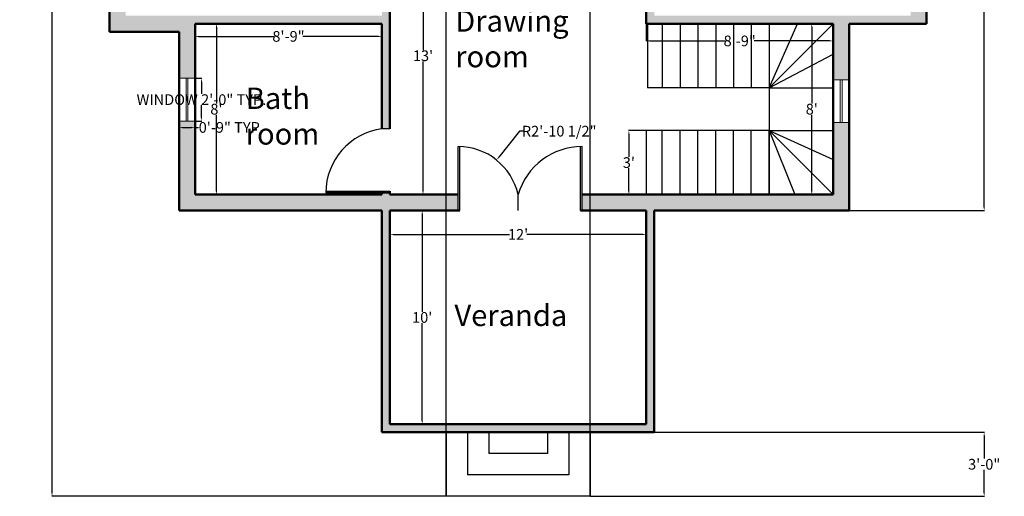
# Model space of a CAD drawing. Units: inches. Extents: x 2436 to 2989, y 5527 to 6207.
# Tile 1 of 5: x 2436 to 2989, y 5527 to 5794. Entities that reach past the tile are written whole.
import ezdxf

# ---------------------------------------------------------------- set-up
doc = ezdxf.new("R2010")
doc.units = ezdxf.units.IN
doc.header["$MEASUREMENT"] = 0
for name, color, linetype, lineweight in [('A-ANNO-DIMS', 2, 'Continuous', 18), ('A-AREA-IDEN', 7, 'Continuous', 25), ('A-DOOR', 3, 'Continuous', 25), ('A-FLOR-STRS', 7, 'Continuous', 25), ('A-GLAZ', 4, 'Continuous', 18), ('A-WALL', 7, 'Continuous', 50), ('A-WALL-PATT', 252, 'Continuous', 13)]:
    doc.layers.add(name, color=color, linetype=linetype, lineweight=lineweight)
doc.styles.get("Standard").update_dxf_attribs({"font": 'arial.ttf'})
doc.dimstyles.get("Standard").update_dxf_attribs({"dimtxt": 6, "dimasz": 2, "dimexe": 0.18, "dimexo": 0.0625, "dimgap": 0.09, "dimtad": 0, "dimtih": 1, "dimtoh": 1, "dimdec": 0, "dimzin": 0, "dimdsep": 46, "dimlunit": 3, "dimtxsty": 'Standard', "dimcen": 0.09, "dimadec": 0, "dimazin": 0, "dimtfac": 1, "dimtdec": 0, "dimtofl": 0, "dimtmove": 0, "dimatfit": 3, "dimfxl": 1, "dimtolj": 1, "dimtzin": 0, "dimarcsym": 0})

# ---------------------------------------------------------------- blocks, each defined once
blk = doc.blocks.new('*D9')
at = {"layer": 'A-ANNO-DIMS', "color": 0, "lineweight": -2, "transparency": 16777216}
for p, q in [((2534.45, 5792.23), (2546.57, 5792.23)), ((2546.39, 5790.23), (2546.39, 5747.39)), ((2546.39, 5698.23), (2546.39, 5741.08)), ((2534.45, 5696.23), (2546.57, 5696.23))]:
    blk.add_line(p, q, dxfattribs=at)
at = {"layer": 'A-ANNO-DIMS', "color": 0, "transparency": 16777216}
for points in [[(2546.05, 5790.23), (2546.72, 5790.23), (2546.39, 5792.23)], [(2546.05, 5698.23), (2546.72, 5698.23), (2546.39, 5696.23)]]:
    blk.add_solid(points, dxfattribs=at)
at = {"layer": 'Defpoints', "color": 0, "transparency": 16777216}
for p in [(2534.39, 5792.23), (2534.39, 5696.23), (2546.39, 5696.23)]:
    blk.add_point(p, dxfattribs=at)
at = {"layer": 'A-ANNO-DIMS', "color": 0, "transparency": 16777216, "insert": (2546.39, 5744.23), "char_height": 6, "attachment_point": 5}
blk.add_mtext("\\A1;8'", dxfattribs=at)
blk = doc.blocks.new('*D10')
at = {"layer": 'A-ANNO-DIMS', "color": 0, "lineweight": -2, "transparency": 16777216}
for p, q in [((2534.39, 5792.17), (2534.39, 5784.93)), ((2639.39, 5792.17), (2639.39, 5784.93)), ((2536.39, 5785.11), (2578.82, 5785.11)), ((2637.39, 5785.11), (2594.96, 5785.11))]:
    blk.add_line(p, q, dxfattribs=at)
at = {"layer": 'A-ANNO-DIMS', "color": 0, "transparency": 16777216}
for points in [[(2536.39, 5785.44), (2536.39, 5784.77), (2534.39, 5785.11)], [(2637.39, 5785.44), (2637.39, 5784.77), (2639.39, 5785.11)]]:
    blk.add_solid(points, dxfattribs=at)
at = {"layer": 'Defpoints', "color": 0, "transparency": 16777216}
for p in [(2534.39, 5792.23), (2639.39, 5792.23), (2639.39, 5785.11)]:
    blk.add_point(p, dxfattribs=at)
at = {"layer": 'A-ANNO-DIMS', "color": 0, "transparency": 16777216, "insert": (2586.89, 5785.11), "char_height": 6, "width": 15.9577, "attachment_point": 5}
blk.add_mtext('\\A1;8\'-9"', dxfattribs=at)
blk = doc.blocks.new('*D11')
at = {"layer": 'A-ANNO-DIMS', "color": 0, "lineweight": -2, "transparency": 16777216}
for p, q in [((2787.89, 5792.17), (2787.89, 5782.38)), ((2892.89, 5792.17), (2892.89, 5782.38)), ((2789.89, 5782.56), (2832.32, 5782.56)), ((2890.89, 5782.56), (2848.46, 5782.56))]:
    blk.add_line(p, q, dxfattribs=at)
at = {"layer": 'A-ANNO-DIMS', "color": 0, "transparency": 16777216}
for points in [[(2789.89, 5782.9), (2789.89, 5782.23), (2787.89, 5782.56)], [(2890.89, 5782.9), (2890.89, 5782.23), (2892.89, 5782.56)]]:
    blk.add_solid(points, dxfattribs=at)
at = {"layer": 'Defpoints', "color": 0, "transparency": 16777216}
for p in [(2787.89, 5792.23), (2892.89, 5792.23), (2892.89, 5782.56)]:
    blk.add_point(p, dxfattribs=at)
at = {"layer": 'A-ANNO-DIMS', "color": 0, "transparency": 16777216, "insert": (2840.39, 5782.56), "char_height": 6, "width": 15.9577, "attachment_point": 5}
blk.add_mtext('\\A1;8\'-9"', dxfattribs=at)
blk = doc.blocks.new('*D12')
at = {"layer": 'A-ANNO-DIMS', "color": 0, "lineweight": -2, "transparency": 16777216}
for p, q in [((2892.83, 5792.23), (2880.71, 5792.23)), ((2880.89, 5790.23), (2880.89, 5747.39)), ((2880.89, 5698.23), (2880.89, 5741.08)), ((2892.83, 5696.23), (2880.71, 5696.23))]:
    blk.add_line(p, q, dxfattribs=at)
at = {"layer": 'A-ANNO-DIMS', "color": 0, "transparency": 16777216}
for points in [[(2880.55, 5790.23), (2881.22, 5790.23), (2880.89, 5792.23)], [(2880.55, 5698.23), (2881.22, 5698.23), (2880.89, 5696.23)]]:
    blk.add_solid(points, dxfattribs=at)
at = {"layer": 'Defpoints', "color": 0, "transparency": 16777216}
for p in [(2892.89, 5792.23), (2880.89, 5696.23), (2892.89, 5696.23)]:
    blk.add_point(p, dxfattribs=at)
at = {"layer": 'A-ANNO-DIMS', "color": 0, "transparency": 16777216, "insert": (2880.89, 5744.23), "char_height": 6, "attachment_point": 5}
blk.add_mtext("\\A1;8'", dxfattribs=at)
blk = doc.blocks.new('*D13')
at = {"layer": 'A-ANNO-DIMS', "color": 0, "lineweight": -2, "transparency": 16777216}
for p, q in [((2643.95, 5852.23), (2662.66, 5852.23)), ((2662.48, 5850.23), (2662.48, 5777.39)), ((2662.48, 5698.23), (2662.48, 5771.08)), ((2643.95, 5696.23), (2662.66, 5696.23))]:
    blk.add_line(p, q, dxfattribs=at)
at = {"layer": 'A-ANNO-DIMS', "color": 0, "transparency": 16777216}
for points in [[(2662.15, 5850.23), (2662.81, 5850.23), (2662.48, 5852.23)], [(2662.15, 5698.23), (2662.81, 5698.23), (2662.48, 5696.23)]]:
    blk.add_solid(points, dxfattribs=at)
at = {"layer": 'Defpoints', "color": 0, "transparency": 16777216}
for p in [(2643.89, 5852.23), (2643.89, 5696.23), (2662.48, 5696.23)]:
    blk.add_point(p, dxfattribs=at)
at = {"layer": 'A-ANNO-DIMS', "color": 0, "transparency": 16777216, "insert": (2662.48, 5774.23), "char_height": 6, "attachment_point": 5}
blk.add_mtext("\\A1;13'", dxfattribs=at)
blk = doc.blocks.new('*D17')
at = {"layer": 'A-ANNO-DIMS', "color": 0, "lineweight": -2, "transparency": 16777216}
for p, q in [((2643.89, 5687.17), (2643.89, 5673.69)), ((2787.89, 5687.17), (2787.89, 5673.69)), ((2645.89, 5673.87), (2710.99, 5673.87)), ((2785.89, 5673.87), (2720.79, 5673.87))]:
    blk.add_line(p, q, dxfattribs=at)
at = {"layer": 'A-ANNO-DIMS', "color": 0, "transparency": 16777216}
for points in [[(2645.89, 5674.2), (2645.89, 5673.53), (2643.89, 5673.87)], [(2785.89, 5674.2), (2785.89, 5673.53), (2787.89, 5673.87)]]:
    blk.add_solid(points, dxfattribs=at)
at = {"layer": 'Defpoints', "color": 0, "transparency": 16777216}
for p in [(2643.89, 5687.23), (2787.89, 5687.23), (2787.89, 5673.87)]:
    blk.add_point(p, dxfattribs=at)
at = {"layer": 'A-ANNO-DIMS', "color": 0, "transparency": 16777216, "insert": (2715.89, 5673.87), "char_height": 6, "attachment_point": 5}
blk.add_mtext("\\A1;12'", dxfattribs=at)
blk = doc.blocks.new('*D18')
at = {"layer": 'A-ANNO-DIMS', "color": 0, "lineweight": -2, "transparency": 16777216}
for p, q in [((2643.95, 5687.23), (2662.19, 5687.23)), ((2662.01, 5685.23), (2662.01, 5630.39)), ((2662.01, 5569.23), (2662.01, 5624.08)), ((2643.95, 5567.23), (2662.19, 5567.23))]:
    blk.add_line(p, q, dxfattribs=at)
at = {"layer": 'A-ANNO-DIMS', "color": 0, "transparency": 16777216}
for points in [[(2661.68, 5685.23), (2662.34, 5685.23), (2662.01, 5687.23)], [(2661.68, 5569.23), (2662.34, 5569.23), (2662.01, 5567.23)]]:
    blk.add_solid(points, dxfattribs=at)
at = {"layer": 'Defpoints', "color": 0, "transparency": 16777216}
for p in [(2643.89, 5687.23), (2643.89, 5567.23), (2662.01, 5567.23)]:
    blk.add_point(p, dxfattribs=at)
at = {"layer": 'A-ANNO-DIMS', "color": 0, "transparency": 16777216, "insert": (2662.01, 5627.23), "char_height": 6, "attachment_point": 5}
blk.add_mtext("\\A1;10'", dxfattribs=at)
blk = doc.blocks.new('*D26')
at = {"layer": 'A-ANNO-DIMS', "color": 0, "lineweight": -2, "transparency": 16777216}
for p, q in [((2787.95, 5732.23), (2777.95, 5732.23)), ((2778.13, 5730.23), (2778.13, 5717.39)), ((2778.13, 5698.23), (2778.13, 5711.08)), ((2787.95, 5696.23), (2777.95, 5696.23))]:
    blk.add_line(p, q, dxfattribs=at)
at = {"layer": 'A-ANNO-DIMS', "color": 0, "transparency": 16777216}
for points in [[(2777.8, 5730.23), (2778.47, 5730.23), (2778.13, 5732.23)], [(2777.8, 5698.23), (2778.47, 5698.23), (2778.13, 5696.23)]]:
    blk.add_solid(points, dxfattribs=at)
at = {"layer": 'Defpoints', "color": 0, "transparency": 16777216}
for p in [(2788.02, 5732.23), (2778.13, 5696.23), (2788.02, 5696.23)]:
    blk.add_point(p, dxfattribs=at)
at = {"layer": 'A-ANNO-DIMS', "color": 0, "transparency": 16777216, "insert": (2778.13, 5714.23), "char_height": 6, "attachment_point": 5}
blk.add_mtext("\\A1;3'", dxfattribs=at)
blk = doc.blocks.new('WINDOW-24IN')
for p, q in [((0, 24), (9, 24)), ((0, 0), (0, 24)), ((4, 0), (4, 24)), ((5, 24), (5, 0)), ((9, 24), (9, 0)), ((9, 0), (0, 0))]:
    blk.add_line(p, q)
blk = doc.blocks.new('DOOR-SWING-36IN')
for p, q in [((1, 0), (1, 36)), ((1, 36), (1, 0)), ((2, 36), (2, 0)), ((0, 0), (1, 0)), ((1, 0), (2, 0)), ((37, 0), (37, 4.5))]:
    blk.add_line(p, q)
blk.add_arc((1, -0.32), 36.32, 7.6281, 90)
blk = doc.blocks.new('*D42')
at = {"layer": 'A-ANNO-DIMS', "color": 0, "lineweight": -2, "transparency": 16777216}
for p, q in [((2534.45, 5761.57), (2538.17, 5761.57)), ((2537.99, 5759.57), (2537.99, 5752.76)), ((2537.99, 5739.57), (2537.99, 5746.38)), ((2534.45, 5737.57), (2538.17, 5737.57))]:
    blk.add_line(p, q, dxfattribs=at)
at = {"layer": 'A-ANNO-DIMS', "color": 0, "transparency": 16777216}
for points in [[(2537.65, 5759.57), (2538.32, 5759.57), (2537.99, 5761.57)], [(2537.65, 5739.57), (2538.32, 5739.57), (2537.99, 5737.57)]]:
    blk.add_solid(points, dxfattribs=at)
at = {"layer": 'Defpoints', "color": 0, "transparency": 16777216}
for p in [(2534.39, 5761.57), (2537.99, 5761.57), (2534.39, 5737.57)]:
    blk.add_point(p, dxfattribs=at)
at = {"layer": 'A-ANNO-DIMS', "color": 0, "transparency": 16777216, "insert": (2537.99, 5749.57), "char_height": 6, "attachment_point": 5}
blk.add_mtext('\\A1;WINDOW 2\'-0" TYP.', dxfattribs=at)
blk = doc.blocks.new('*D43')
at = {"layer": 'A-ANNO-DIMS', "color": 0, "lineweight": -2, "transparency": 16777216}
for p, q in [((2525.39, 5737.51), (2525.39, 5733.79)), ((2534.39, 5737.51), (2534.39, 5733.79)), ((2527.39, 5733.97), (2532.39, 5733.97)), ((2534.39, 5733.97), (2536.39, 5733.97))]:
    blk.add_line(p, q, dxfattribs=at)
at = {"layer": 'A-ANNO-DIMS', "color": 0, "transparency": 16777216}
for points in [[(2527.39, 5734.3), (2527.39, 5733.64), (2525.39, 5733.97)], [(2532.39, 5734.3), (2532.39, 5733.64), (2534.39, 5733.97)]]:
    blk.add_solid(points, dxfattribs=at)
at = {"layer": 'Defpoints', "color": 0, "transparency": 16777216}
for p in [(2525.39, 5737.57), (2534.39, 5737.57), (2534.39, 5733.97)]:
    blk.add_point(p, dxfattribs=at)
at = {"layer": 'A-ANNO-DIMS', "color": 0, "transparency": 16777216, "insert": (2554.76, 5733.97), "char_height": 6, "attachment_point": 5}
blk.add_mtext('\\A1;0\'-9" TYP.', dxfattribs=at)
blk = doc.blocks.new('*D49')
at = {"layer": 'A-ANNO-DIMS', "color": 0, "lineweight": -2, "transparency": 16777216}
for p, q in [((2486.33, 6170.23), (2453.86, 6170.23)), ((2454.04, 6168.23), (2454.04, 5851.68)), ((2454.04, 5528.73), (2454.04, 5845.29)), ((2675.33, 5526.73), (2453.86, 5526.73))]:
    blk.add_line(p, q, dxfattribs=at)
at = {"layer": 'A-ANNO-DIMS', "color": 0, "transparency": 16777216}
for points in [[(2453.7, 6168.23), (2454.37, 6168.23), (2454.04, 6170.23)], [(2453.7, 5528.73), (2454.37, 5528.73), (2454.04, 5526.73)]]:
    blk.add_solid(points, dxfattribs=at)
at = {"layer": 'Defpoints', "color": 0, "transparency": 16777216}
for p in [(2486.39, 6170.23), (2454.04, 5526.73), (2675.39, 5526.73)]:
    blk.add_point(p, dxfattribs=at)
at = {"layer": 'A-ANNO-DIMS', "color": 0, "transparency": 16777216, "insert": (2454.04, 5848.48), "char_height": 6, "attachment_point": 5}
blk.add_mtext('\\A1;53\'-7 1/2"', dxfattribs=at)
blk = doc.blocks.new('*D50')
at = {"layer": 'A-ANNO-DIMS', "color": 0, "lineweight": -2, "transparency": 16777216}
for p, q in [((2792.45, 6170.23), (2977.92, 6170.23)), ((2977.74, 6168.23), (2977.74, 5931.89)), ((2977.74, 5689.23), (2977.74, 5925.58)), ((2901.95, 5687.23), (2977.92, 5687.23))]:
    blk.add_line(p, q, dxfattribs=at)
at = {"layer": 'A-ANNO-DIMS', "color": 0, "transparency": 16777216}
for points in [[(2977.4, 6168.23), (2978.07, 6168.23), (2977.74, 6170.23)], [(2977.4, 5689.23), (2978.07, 5689.23), (2977.74, 5687.23)]]:
    blk.add_solid(points, dxfattribs=at)
at = {"layer": 'Defpoints', "color": 0, "transparency": 16777216}
for p in [(2792.39, 6170.23), (2901.89, 5687.23), (2977.74, 5687.23)]:
    blk.add_point(p, dxfattribs=at)
at = {"layer": 'A-ANNO-DIMS', "color": 0, "transparency": 16777216, "insert": (2977.74, 5928.73), "char_height": 6, "attachment_point": 5}
blk.add_mtext('\\A1;40\'-3"', dxfattribs=at)
blk = doc.blocks.new('*D51')
at = {"layer": 'A-ANNO-DIMS', "color": 0, "lineweight": -2, "transparency": 16777216}
for p, q in [((2675.39, 5526.79), (2675.39, 6202.76)), ((2677.39, 6202.58), (2707.81, 6202.58)), ((2754.39, 6202.58), (2723.97, 6202.58)), ((2756.39, 5526.79), (2756.39, 6202.76))]:
    blk.add_line(p, q, dxfattribs=at)
at = {"layer": 'A-ANNO-DIMS', "color": 0, "transparency": 16777216}
for points in [[(2677.39, 6202.92), (2677.39, 6202.25), (2675.39, 6202.58)], [(2754.39, 6202.92), (2754.39, 6202.25), (2756.39, 6202.58)]]:
    blk.add_solid(points, dxfattribs=at)
at = {"layer": 'Defpoints', "color": 0, "transparency": 16777216}
for p in [(2756.39, 6202.58), (2675.39, 5526.73), (2756.39, 5526.73)]:
    blk.add_point(p, dxfattribs=at)
at = {"layer": 'A-ANNO-DIMS', "color": 0, "transparency": 16777216, "insert": (2715.89, 6202.58), "char_height": 6, "attachment_point": 5}
blk.add_mtext('\\A1;6\'-9"', dxfattribs=at)
blk = doc.blocks.new('*D52')
at = {"layer": 'A-ANNO-DIMS', "color": 0, "lineweight": -2, "transparency": 16777216}
for p, q in [((2756.45, 5562.73), (2977.92, 5562.73)), ((2977.74, 5560.73), (2977.74, 5547.89)), ((2977.74, 5528.73), (2977.74, 5541.58)), ((2756.45, 5526.73), (2977.92, 5526.73))]:
    blk.add_line(p, q, dxfattribs=at)
at = {"layer": 'A-ANNO-DIMS', "color": 0, "transparency": 16777216}
for points in [[(2977.4, 5560.73), (2978.07, 5560.73), (2977.74, 5562.73)], [(2977.4, 5528.73), (2978.07, 5528.73), (2977.74, 5526.73)]]:
    blk.add_solid(points, dxfattribs=at)
at = {"layer": 'Defpoints', "color": 0, "transparency": 16777216}
for p in [(2756.39, 5562.73), (2756.39, 5526.73), (2977.74, 5526.73)]:
    blk.add_point(p, dxfattribs=at)
at = {"layer": 'A-ANNO-DIMS', "color": 0, "transparency": 16777216, "insert": (2977.74, 5544.73), "char_height": 6, "attachment_point": 5}
blk.add_mtext('\\A1;3\'-0"', dxfattribs=at)
blk = doc.blocks.new('*D53')
at = {"layer": 'A-ANNO-DIMS', "color": 0, "lineweight": -2, "transparency": 16777216}
for p, q in [((2716.72, 5731.86), (2705, 5717.21)), ((2718.72, 5731.86), (2716.72, 5731.86)), ((2682.05, 5688.64), (2682.23, 5688.64)), ((2682.14, 5688.55), (2682.14, 5688.73))]:
    blk.add_line(p, q, dxfattribs=at)
at = {"layer": 'A-ANNO-DIMS', "color": 0, "transparency": 16777216}
blk.add_solid([(2704.74, 5717.42), (2705.26, 5717.01), (2703.75, 5715.65)], dxfattribs=at)
at = {"layer": 'Defpoints', "color": 0, "transparency": 16777216}
for p in [(2703.75, 5715.65), (2682.14, 5688.64)]:
    blk.add_point(p, dxfattribs=at)
at = {"layer": 'A-ANNO-DIMS', "color": 0, "transparency": 16777216, "insert": (2738.97, 5731.86), "char_height": 6, "attachment_point": 5}
blk.add_mtext('\\A1;R2\'-10 1/2"', dxfattribs=at)

msp = doc.modelspace()

# ---------------------------------------------------------------- hatches: boundary and pattern name
at = {"layer": 'A-WALL-PATT'}
h = msp.add_hatch(color=256, dxfattribs=at)
h.dxf.hatch_style = 1
h.paths.add_polyline_path([(2533.49, 6170.23), (2486.39, 6170.23), (2486.39, 6124.33), (2495.39, 6124.33), (2495.39, 6161.23), (2533.49, 6161.23)])
h.paths.add_polyline_path([(2677.58, 6170.23), (2593.49, 6170.23), (2593.49, 6161.23), (2639.39, 6161.23), (2639.39, 6035.73), (2639.39, 6035.73), (2643.89, 6035.73), (2643.89, 6036.73), (2685.89, 6036.73), (2685.89, 6041.23), (2643.89, 6041.23), (2643.89, 6161.23), (2677.58, 6161.23)])
h.paths.add_polyline_path([(2792.39, 6170.23), (2737.58, 6170.23), (2737.58, 6161.23), (2787.89, 6161.23), (2787.89, 6084.23), (2792.39, 6084.23), (2792.39, 6161.23), (2936.39, 6161.23), (2936.39, 6071.23), (2840.39, 6071.23), (2840.39, 6047.23), (2792.39, 6047.23), (2792.39, 6048.23), (2787.89, 6048.23), (2787.89, 6047.23), (2787.89, 6041.23), (2742.3, 6041.23), (2742.3, 6036.73), (2787.89, 6036.73), (2787.89, 6035.73), (2792.39, 6035.73), (2792.39, 6042.73), (2840.39, 6042.73), (2840.39, 5945.23), (2792.39, 5945.23), (2792.39, 6003.73), (2787.89, 6003.73), (2787.89, 5893.73), (2792.39, 5893.73), (2792.39, 5940.73), (2845.89, 5940.73), (2845.89, 5945.23), (2844.89, 5945.23), (2844.89, 6047.23), (2844.89, 6066.73), (2936.39, 6066.73), (2936.39, 6024.33), (2945.39, 6024.33), (2945.39, 6080.66), (2940.89, 6080.66), (2940.89, 6165.73), (2792.39, 6165.73)])
h.paths.add_polyline_path([(2945.39, 6000.33), (2936.39, 6000.33), (2936.39, 5945.23), (2881.89, 5945.23), (2881.89, 5940.73), (2936.39, 5940.73), (2936.39, 5901.74), (2945.39, 5901.74)], flags=17)
h.paths.add_polyline_path([(2945.39, 5841.74), (2936.39, 5841.74), (2936.39, 5796.73), (2792.39, 5796.73), (2792.39, 5857.73), (2787.89, 5857.73), (2787.89, 5856.73), (2786.89, 5856.73), (2786.89, 5852.23), (2787.89, 5852.23), (2787.89, 5792.23), (2892.89, 5792.23), (2892.89, 5760.78), (2901.89, 5760.78), (2901.89, 5792.23), (2945.39, 5792.23)])
h.paths.add_polyline_path([(2495.39, 5880.74), (2486.39, 5880.74), (2486.39, 5787.73), (2525.39, 5787.73), (2525.39, 5761.57), (2534.39, 5761.57), (2534.39, 5792.23), (2639.39, 5792.23), (2639.39, 5733.23), (2643.89, 5733.23), (2643.89, 5852.23), (2750.89, 5852.23), (2750.89, 5856.73), (2643.89, 5856.73), (2643.89, 5857.73), (2639.39, 5857.73), (2639.39, 5796.73), (2495.39, 5796.73)])
h.paths.add_polyline_path([(2495.39, 6064.33), (2486.39, 6064.33), (2486.39, 5940.74), (2495.39, 5940.74), (2495.39, 5988.73), (2639.39, 5988.73), (2639.39, 5893.73), (2643.89, 5893.73), (2643.89, 5999.73), (2639.39, 5999.73), (2639.39, 5993.23), (2495.39, 5993.23)])
h.paths.add_polyline_path([(2682.14, 5696.23), (2643.89, 5696.23), (2643.89, 5697.23), (2639.39, 5697.23), (2639.39, 5696.23), (2558.39, 5696.23), (2534.39, 5696.23), (2534.39, 5737.57), (2525.39, 5737.57), (2525.39, 5687.23), (2534.39, 5687.23), (2558.39, 5687.23), (2643.89, 5687.23), (2682.14, 5687.23)])
h.paths.add_polyline_path([(2901.89, 5736.78), (2892.89, 5736.78), (2892.89, 5696.23), (2868.89, 5696.23), (2751.89, 5696.23), (2751.89, 5687.23), (2787.89, 5687.23), (2787.89, 5567.23), (2792.39, 5567.23), (2792.39, 5687.23), (2868.89, 5687.23), (2892.89, 5687.23), (2901.89, 5687.23)])
h.paths.add_polyline_path([(2643.89, 5687.23), (2639.39, 5687.23), (2639.39, 5567.23), (2643.89, 5567.23)])
h.paths.add_polyline_path([(2787.89, 5567.23), (2643.89, 5567.23), (2643.89, 5562.73), (2787.89, 5562.73)])
h.paths.add_polyline_path([(2643.89, 5567.23), (2639.39, 5567.23), (2639.39, 5562.73), (2643.89, 5562.73)])
h.paths.add_polyline_path([(2792.39, 5567.23), (2787.89, 5567.23), (2787.89, 5562.73), (2792.39, 5562.73)])

# ---------------------------------------------------------------- linework, layer by layer
at = {"layer": 'A-DOOR'}
for p, q in [((2682.14, 5687.23), (2682.14, 5723.23)), ((2683.14, 5687.23), (2683.14, 5723.23)), ((2750.89, 5687.23), (2750.89, 5723.23)), ((2751.89, 5687.23), (2751.89, 5723.23)), ((2643.89, 5697.23), (2643.89, 5697.23)), ((2715.89, 5687.23), (2715.89, 5696.23)), ((2683.14, 5687.23), (2682.14, 5687.23)), ((2750.89, 5687.23), (2751.89, 5687.23))]:
    msp.add_line(p, q, dxfattribs=at)
for centre, radius, start, end in [((2682.14, 5688.64), 34.59, 12.6804, 90), ((2751.89, 5685.73), 37.5, 90, 163.7398)]:
    msp.add_arc(centre, radius, start, end, dxfattribs=at)
at = {"layer": 'A-FLOR-STRS'}
for p, q in [((2788.54, 5792.23), (2788.54, 5756.23)), ((2796.89, 5792.23), (2796.89, 5756.23)), ((2806.89, 5792.23), (2806.89, 5756.23)), ((2816.89, 5792.23), (2816.89, 5756.23)), ((2859.89, 5792.23), (2823.89, 5792.23)), ((2826.89, 5792.23), (2826.89, 5756.23)), ((2836.89, 5792.23), (2836.89, 5756.23)), ((2846.89, 5792.23), (2846.89, 5756.23)), ((2892.89, 5792.23), (2856.89, 5792.23)), ((2856.89, 5792.23), (2856.89, 5696.23)), ((2856.89, 5792.23), (2856.89, 5756.23)), ((2856.89, 5756.23), (2892.89, 5792.23)), ((2856.89, 5756.23), (2872.92, 5792.23)), ((2856.89, 5756.23), (2892.89, 5775.18)), ((2856.89, 5756.23), (2788.54, 5756.23)), ((2856.89, 5756.23), (2892.89, 5756.23)), ((2856.89, 5732.23), (2788.02, 5732.23)), ((2788.02, 5696.23), (2788.02, 5732.23)), ((2796.89, 5696.23), (2796.89, 5732.23)), ((2806.89, 5696.23), (2806.89, 5732.23)), ((2816.89, 5696.23), (2816.89, 5732.23)), ((2826.89, 5696.23), (2826.89, 5732.23)), ((2836.89, 5696.23), (2836.89, 5732.23)), ((2846.89, 5696.23), (2846.89, 5732.23)), ((2856.89, 5696.23), (2856.89, 5732.23)), ((2856.89, 5732.23), (2892.89, 5732.23)), ((2856.89, 5732.23), (2892.89, 5696.23)), ((2856.89, 5732.23), (2892.89, 5715.88)), ((2856.89, 5732.23), (2871.34, 5696.23)), ((2639.39, 5562.73), (2675.39, 5562.73)), ((2675.39, 5562.73), (2675.39, 5526.73)), ((2687.39, 5562.73), (2687.39, 5538.73)), ((2699.39, 5562.73), (2699.39, 5550.73)), ((2732.39, 5562.73), (2732.39, 5550.73)), ((2744.39, 5562.73), (2744.39, 5538.73)), ((2792.39, 5562.73), (2756.39, 5562.73)), ((2756.39, 5562.73), (2756.39, 5526.73)), ((2732.39, 5550.73), (2699.39, 5550.73)), ((2744.39, 5538.73), (2687.39, 5538.73)), ((2756.39, 5526.73), (2675.39, 5526.73))]:
    msp.add_line(p, q, dxfattribs=at)
at = {"layer": 'A-WALL'}
for p, q in [((2486.39, 6170.23), (2486.39, 5787.73)), ((2945.39, 6080.66), (2945.39, 5792.23)), ((2643.89, 5852.23), (2643.89, 5733.23)), ((2787.89, 5852.23), (2787.89, 5792.23)), ((2534.39, 5792.23), (2639.39, 5792.23)), ((2534.39, 5696.23), (2534.39, 5792.23)), ((2639.39, 5792.23), (2639.39, 5733.23)), ((2787.89, 5792.23), (2892.89, 5792.23)), ((2892.89, 5696.23), (2892.89, 5792.23)), ((2901.89, 5687.23), (2901.89, 5792.23)), ((2901.89, 5792.23), (2945.39, 5792.23)), ((2486.39, 5787.73), (2525.39, 5787.73)), ((2525.39, 5687.23), (2525.39, 5787.73)), ((2643.89, 5698.23), (2643.89, 5696.23)), ((2558.39, 5696.23), (2534.39, 5696.23)), ((2558.39, 5696.23), (2567.39, 5696.23)), ((2567.39, 5696.23), (2639.39, 5696.23)), ((2639.39, 5697.23), (2639.39, 5696.23)), ((2643.89, 5696.23), (2682.14, 5696.23)), ((2751.89, 5696.23), (2868.89, 5696.23)), ((2868.89, 5696.23), (2892.89, 5696.23)), ((2534.39, 5687.23), (2525.39, 5687.23)), ((2558.39, 5687.23), (2534.39, 5687.23)), ((2558.39, 5687.23), (2567.39, 5687.23)), ((2567.39, 5687.23), (2639.39, 5687.23)), ((2639.39, 5687.23), (2639.39, 5562.73)), ((2643.89, 5687.23), (2643.89, 5567.23)), ((2643.89, 5687.23), (2683.14, 5687.23)), ((2750.89, 5687.23), (2787.89, 5687.23)), ((2750.89, 5687.23), (2787.89, 5687.23)), ((2787.89, 5687.23), (2787.89, 5567.23)), ((2792.39, 5687.23), (2792.39, 5562.73)), ((2792.39, 5687.23), (2868.89, 5687.23)), ((2868.89, 5687.23), (2892.89, 5687.23)), ((2892.89, 5687.23), (2901.89, 5687.23)), ((2643.89, 5567.23), (2787.89, 5567.23)), ((2639.39, 5562.73), (2792.39, 5562.73))]:
    msp.add_line(p, q, dxfattribs=at)

# ---------------------------------------------------------------- block references
at = {"layer": 'A-DOOR', "rotation": 89.9999999999965}
msp.add_blockref('DOOR-SWING-36IN', (2643.89, 5696.23), dxfattribs=at)
at = {"layer": 'A-GLAZ'}
msp.add_blockref('WINDOW-24IN', (2525.39, 5737.57), dxfattribs=at)
at = {"layer": 'A-GLAZ', "rotation": 180}
msp.add_blockref('WINDOW-24IN', (2901.89, 5760.78), dxfattribs=at)

# ---------------------------------------------------------------- texts
at = {"layer": 'A-AREA-IDEN', "char_height": 12, "attachment_point": 1}
for s, width, insert in [('Drawing\\Proom', 69.5872, (2680.57, 5799.76)), ('Bath\\Proom', 56.1363, (2562.85, 5756.33)), ('Veranda', 80.3465, (2680.12, 5634.38))]:
    msp.add_mtext_dynamic_manual_height_columns(s, width=width, gutter_width=1, heights=[0], dxfattribs=dict(at, insert=insert))

# ---------------------------------------------------------------- dimensions: what is measured, and where the dimension line sits
at = {"layer": 'A-ANNO-DIMS'}
for base, p1, p2, override, picture, middle in [((2756.39, 6202.58), (2675.39, 5526.73), (2756.39, 5526.73), {"dimdec": 1, "dimlfac": 1, "dimrnd": 0, "dimzin": 1, "dimdsep": 46, "dimlunit": 4, "dimfrac": 2}, '*D51', (2715.89, 6202.58)), ((2639.39, 5785.11), (2534.39, 5792.23), (2639.39, 5792.23), {"dimclrd": 0, "dimclre": 0, "dimclrt": 0}, '*D10', (2586.89, 5785.11)), ((2892.89, 5782.56), (2787.89, 5792.23), (2892.89, 5792.23), {"dimclrd": 0, "dimclre": 0, "dimclrt": 0}, '*D11', (2840.39, 5782.56)), ((2787.89, 5673.87), (2643.89, 5687.23), (2787.89, 5687.23), {"dimclrd": 0, "dimclre": 0, "dimclrt": 0}, '*D17', (2715.89, 5673.87))]:
    dim = msp.add_linear_dim(base=base, p1=p1, p2=p2, dimstyle='Standard', override=override, dxfattribs=at)
    dim.commit()
    dim.dimension.update_dxf_attribs({"geometry": picture, "text_midpoint": middle})
for base, p1, p2, override, picture, middle in [((2454.04, 5526.73), (2486.39, 6170.23), (2675.39, 5526.73), {"dimdec": 1, "dimlfac": 1, "dimrnd": 0, "dimzin": 1, "dimdsep": 46, "dimlunit": 4, "dimfrac": 2}, '*D49', (2454.04, 5848.48)), ((2977.74, 5687.23), (2792.39, 6170.23), (2901.89, 5687.23), {"dimdec": 1, "dimlfac": 1, "dimrnd": 0, "dimzin": 1, "dimdsep": 46, "dimlunit": 4, "dimfrac": 2}, '*D50', (2977.74, 5928.73)), ((2662.48, 5696.23), (2643.89, 5852.23), (2643.89, 5696.23), {"dimclrd": 0, "dimclre": 0, "dimclrt": 0}, '*D13', (2662.48, 5774.23)), ((2546.39, 5696.23), (2534.39, 5792.23), (2534.39, 5696.23), {"dimclrd": 0, "dimclre": 0, "dimclrt": 0}, '*D9', (2546.39, 5744.23)), ((2880.89, 5696.23), (2892.89, 5792.23), (2892.89, 5696.23), {"dimclrd": 0, "dimclre": 0, "dimclrt": 0}, '*D12', (2880.89, 5744.23)), ((2778.13, 5696.23), (2788.02, 5732.23), (2788.02, 5696.23), {"dimclrd": 0, "dimclre": 0, "dimclrt": 0}, '*D26', (2778.13, 5714.23)), ((2662.01, 5567.23), (2643.89, 5687.23), (2643.89, 5567.23), {"dimclrd": 0, "dimclre": 0, "dimclrt": 0}, '*D18', (2662.01, 5627.23)), ((2977.74, 5526.73), (2756.39, 5562.73), (2756.39, 5526.73), {"dimdec": 1, "dimlfac": 1, "dimrnd": 0, "dimzin": 1, "dimdsep": 46, "dimlunit": 4, "dimfrac": 2}, '*D52', (2977.74, 5544.73))]:
    dim = msp.add_linear_dim(base=base, p1=p1, p2=p2, angle=90, dimstyle='Standard', override=override, dxfattribs=at)
    dim.commit()
    dim.dimension.update_dxf_attribs({"geometry": picture, "text_midpoint": middle})
dim = msp.add_linear_dim(base=(2537.99, 5761.57), p1=(2534.39, 5737.57), p2=(2534.39, 5761.57), angle=90, text='WINDOW <> TYP.', dimstyle='Standard', override={"dimdec": 1, "dimlfac": 1, "dimrnd": 0, "dimzin": 1, "dimdsep": 46, "dimlunit": 4, "dimfrac": 2}, dxfattribs=at)
dim.commit()
dim.dimension.update_dxf_attribs({"geometry": '*D42', "text_midpoint": (2537.99, 5749.57)})
dim = msp.add_linear_dim(base=(2534.39, 5733.97), p1=(2525.39, 5737.57), p2=(2534.39, 5737.57), text='<> TYP.', dimstyle='Standard', override={"dimdec": 1, "dimlfac": 1, "dimrnd": 0, "dimzin": 1, "dimdsep": 46, "dimlunit": 4, "dimfrac": 2}, dxfattribs=at)
dim.commit()
dim.dimension.update_dxf_attribs({"geometry": '*D43', "text_midpoint": (2554.76, 5733.97)})
dim = msp.add_radius_dim(center=(2682.14, 5688.64), mpoint=(2703.75, 5715.65), dimstyle='Standard', override={"dimdec": 1, "dimlfac": 1, "dimrnd": 0, "dimzin": 1, "dimdsep": 46, "dimlunit": 4, "dimfrac": 2}, dxfattribs=at)
dim.commit()
dim.dimension.update_dxf_attribs({"geometry": '*D53', "text_midpoint": (2738.97, 5731.86), "dimtype": 164})

doc.saveas('drawing.dxf')
